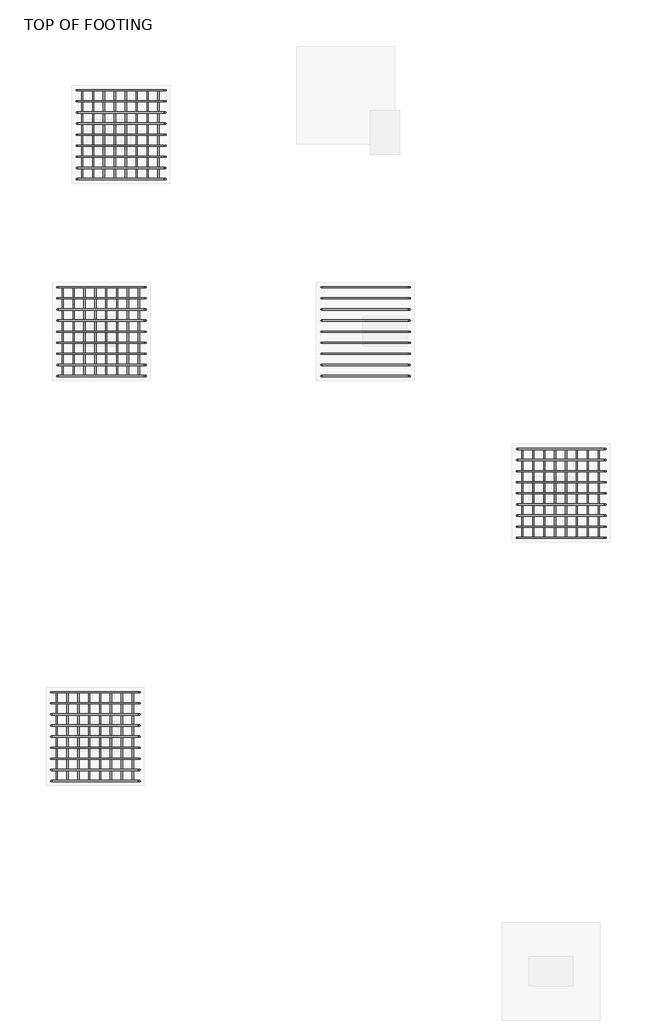
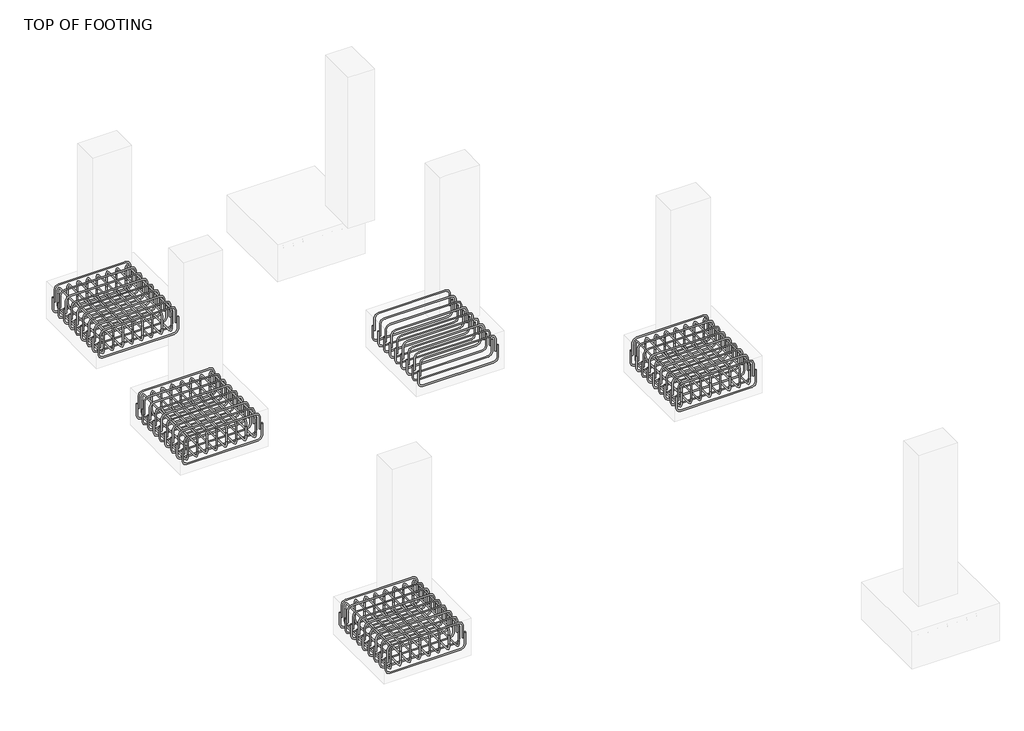
# One storey, part 15 of 20: 18 reinforcing bars.
"""IFC4 building model written with IfcOpenShell, lengths in millimetres."""

from ifc_helpers import new_model, si_unit, point, frame, origin, place, context, project, spatial, polyline, circle_curve, trimmed, segment, composite_curve, source, transform, mapped, element, save
from ifc_brep_helpers import swept_disk

model = new_model("IFC4")

# Units and contexts
model_context = context("Model", 3, world=origin())
ifc_project = project(units=[si_unit("LENGTHUNIT", "METRE", prefix="MILLI")], contexts=[model_context])

# Site, building, storey
site = spatial("IfcSite", under=ifc_project)
building = spatial("IfcBuilding", under=site)
storey = spatial("IfcBuildingStorey", under=building, Name="TOP OF FOOTING", Elevation=-1828.8)

# Reinforcing bars
placement = place(None, origin())
reinforcing_bar_shape = source(origin(), model_context, "Body", "SolidModel", [
    swept_disk(composite_curve([segment(polyline([(10522.7663908, 7703.3576276, -2006.6587682), (10522.7663908, 7703.3576276, -2153.9587682)]), True, "CONTINUOUS"), segment(trimmed(circle_curve(frame((10476.4163908, 7703.3576276, -2153.9587682), z_axis=(0.0, 1.0, 0.0), x_axis=(46.350000000000364, 0.0, 0.0)), 46.35), [point((10522.7663908, 7703.3576276, -2153.9587682))], [point((10476.4163908, 7703.3576276, -2200.3087682))], True, "CARTESIAN"), True, "CONTINUOUS"), segment(polyline([(10476.4163908, 7703.3576276, -2200.3087682), (9661.8163908, 7703.3576276, -2200.3087682)]), True, "CONTINUOUS"), segment(trimmed(circle_curve(frame((9661.8163908, 7703.3576276, -2153.9587682), z_axis=(0.0, 1.0, 0.0), x_axis=(0.0, 0.0, -46.34999999999991)), 46.35), [point((9661.8163908, 7703.3576276, -2200.3087682))], [point((9615.4663908, 7703.3576276, -2153.9587682))], True, "CARTESIAN"), True, "CONTINUOUS"), segment(polyline([(9615.4663908, 7703.3576276, -2153.9587682), (9615.4663908, 7703.3576276, -2006.6587682)]), True, "CONTINUOUS")], self_intersect=False), 6.35),
])
element("IfcReinforcingBar", 1, at=placement, inside=storey, context=model_context, shape_type="MappedRepresentation", body=[
    mapped(reinforcing_bar_shape, transform((0.0, 0.0, 0.0), x_axis=(1.0, 0.0, 0.0), y_axis=(0.0, 1.0, 0.0), z_axis=(0.0, 0.0, 1.0))),
    mapped(reinforcing_bar_shape, transform((0.0, -113.4125, 0.0), x_axis=(1.0, 0.0, 0.0), y_axis=(0.0, 1.0, 0.0), z_axis=(0.0, 0.0, 1.0))),
    mapped(reinforcing_bar_shape, transform((0.0, -226.825, 0.0), x_axis=(1.0, 0.0, 0.0), y_axis=(0.0, 1.0, 0.0), z_axis=(0.0, 0.0, 1.0))),
    mapped(reinforcing_bar_shape, transform((0.0, -340.2375, 0.0), x_axis=(1.0, 0.0, 0.0), y_axis=(0.0, 1.0, 0.0), z_axis=(0.0, 0.0, 1.0))),
    mapped(reinforcing_bar_shape, transform((0.0, -453.65, 0.0), x_axis=(1.0, 0.0, 0.0), y_axis=(0.0, 1.0, 0.0), z_axis=(0.0, 0.0, 1.0))),
    mapped(reinforcing_bar_shape, transform((0.0, -567.0625, 0.0), x_axis=(1.0, 0.0, 0.0), y_axis=(0.0, 1.0, 0.0), z_axis=(0.0, 0.0, 1.0))),
    mapped(reinforcing_bar_shape, transform((0.0, -680.475, 0.0), x_axis=(1.0, 0.0, 0.0), y_axis=(0.0, 1.0, 0.0), z_axis=(0.0, 0.0, 1.0))),
    mapped(reinforcing_bar_shape, transform((0.0, -793.8875, 0.0), x_axis=(1.0, 0.0, 0.0), y_axis=(0.0, 1.0, 0.0), z_axis=(0.0, 0.0, 1.0))),
    mapped(reinforcing_bar_shape, transform((0.0, -907.3, 0.0), x_axis=(1.0, 0.0, 0.0), y_axis=(0.0, 1.0, 0.0), z_axis=(0.0, 0.0, 1.0))),
])
reinforcing_bar_2_shape = source(origin(), model_context, "Body", "SolidModel", [
    swept_disk(composite_curve([segment(polyline([(9634.9405021, 7703.3576276, -2068.8), (9634.9405021, 7703.3576276, -1921.5)]), True, "CONTINUOUS"), segment(trimmed(circle_curve(frame((9681.2905021, 7703.3576276, -1921.5), z_axis=(0.0, 1.0, 0.0), x_axis=(-46.350000000000364, 0.0, 0.0)), 46.35), [point((9634.9405021, 7703.3576276, -1921.5))], [point((9681.2905021, 7703.3576276, -1875.15))], True, "CARTESIAN"), True, "CONTINUOUS"), segment(polyline([(9681.2905021, 7703.3576276, -1875.15), (10450.7539017, 7703.3576276, -1875.15)]), True, "CONTINUOUS"), segment(trimmed(circle_curve(frame((10450.7539017, 7703.3576276, -1921.5), z_axis=(0.0, 1.0, 0.0), x_axis=(0.0, 0.0, 46.34999999999991)), 46.35), [point((10450.7539017, 7703.3576276, -1875.15))], [point((10497.1039017, 7703.3576276, -1921.5))], True, "CARTESIAN"), True, "CONTINUOUS"), segment(polyline([(10497.1039017, 7703.3576276, -1921.5), (10497.1039017, 7703.3576276, -2068.8)]), True, "CONTINUOUS")], self_intersect=False), 6.35),
])
element("IfcReinforcingBar", 2, at=placement, inside=storey, context=model_context, shape_type="MappedRepresentation", body=[
    mapped(reinforcing_bar_2_shape, transform((0.0, 0.0, 0.0), x_axis=(1.0, 0.0, 0.0), y_axis=(0.0, 1.0, 0.0), z_axis=(0.0, 0.0, 1.0))),
    mapped(reinforcing_bar_2_shape, transform((0.0, -113.4125, 0.0), x_axis=(1.0, 0.0, 0.0), y_axis=(0.0, 1.0, 0.0), z_axis=(0.0, 0.0, 1.0))),
    mapped(reinforcing_bar_2_shape, transform((0.0, -226.825, 0.0), x_axis=(1.0, 0.0, 0.0), y_axis=(0.0, 1.0, 0.0), z_axis=(0.0, 0.0, 1.0))),
    mapped(reinforcing_bar_2_shape, transform((0.0, -340.2375, 0.0), x_axis=(1.0, 0.0, 0.0), y_axis=(0.0, 1.0, 0.0), z_axis=(0.0, 0.0, 1.0))),
    mapped(reinforcing_bar_2_shape, transform((0.0, -453.65, 0.0), x_axis=(1.0, 0.0, 0.0), y_axis=(0.0, 1.0, 0.0), z_axis=(0.0, 0.0, 1.0))),
    mapped(reinforcing_bar_2_shape, transform((0.0, -567.0625, 0.0), x_axis=(1.0, 0.0, 0.0), y_axis=(0.0, 1.0, 0.0), z_axis=(0.0, 0.0, 1.0))),
    mapped(reinforcing_bar_2_shape, transform((0.0, -680.475, 0.0), x_axis=(1.0, 0.0, 0.0), y_axis=(0.0, 1.0, 0.0), z_axis=(0.0, 0.0, 1.0))),
    mapped(reinforcing_bar_2_shape, transform((0.0, -793.8875, 0.0), x_axis=(1.0, 0.0, 0.0), y_axis=(0.0, 1.0, 0.0), z_axis=(0.0, 0.0, 1.0))),
    mapped(reinforcing_bar_2_shape, transform((0.0, -907.3, 0.0), x_axis=(1.0, 0.0, 0.0), y_axis=(0.0, 1.0, 0.0), z_axis=(0.0, 0.0, 1.0))),
])
reinforcing_bar_3_shape = source(origin(), model_context, "Body", "SolidModel", [
    swept_disk(composite_curve([segment(polyline([(10451.2694294, 7703.3576276, -2086.1951968), (10451.2694294, 7703.3576276, -1938.8951968)]), True, "CONTINUOUS"), segment(trimmed(circle_curve(frame((10451.2694294, 7657.0076276, -1938.8951968), z_axis=(1.0, 0.0, 0.0), x_axis=(0.0, 46.350000000000364, 0.0)), 46.35), [point((10451.2694294, 7703.3576276, -1938.8951968))], [point((10451.2694294, 7657.0076276, -1892.5451968))], True, "CARTESIAN"), True, "CONTINUOUS"), segment(polyline([(10451.2694294, 7657.0076276, -1892.5451968), (10451.2694294, 6842.4076276, -1892.5451968)]), True, "CONTINUOUS"), segment(trimmed(circle_curve(frame((10451.2694294, 6842.4076276, -1938.8951968), z_axis=(1.0, 0.0, 0.0), x_axis=(0.0, 0.0, 46.34999999999991)), 46.35), [point((10451.2694294, 6842.4076276, -1892.5451968))], [point((10451.2694294, 6796.0576276, -1938.8951968))], True, "CARTESIAN"), True, "CONTINUOUS"), segment(polyline([(10451.2694294, 6796.0576276, -1938.8951968), (10451.2694294, 6796.0576276, -2086.1951968)]), True, "CONTINUOUS")], self_intersect=False), 6.35),
])
element("IfcReinforcingBar", 3, at=placement, inside=storey, context=model_context, shape_type="MappedRepresentation", body=[
    mapped(reinforcing_bar_3_shape, transform((0.0, 0.0, 0.0), x_axis=(1.0, 0.0, 0.0), y_axis=(0.0, 1.0, 0.0), z_axis=(0.0, 0.0, 1.0))),
    mapped(reinforcing_bar_3_shape, transform((-111.2862402, 0.0, 0.0), x_axis=(1.0, 0.0, 0.0), y_axis=(0.0, 1.0, 0.0), z_axis=(0.0, 0.0, 1.0))),
    mapped(reinforcing_bar_3_shape, transform((-222.5724804, 0.0, 0.0), x_axis=(1.0, 0.0, 0.0), y_axis=(0.0, 1.0, 0.0), z_axis=(0.0, 0.0, 1.0))),
    mapped(reinforcing_bar_3_shape, transform((-333.8587205, 0.0, 0.0), x_axis=(1.0, 0.0, 0.0), y_axis=(0.0, 1.0, 0.0), z_axis=(0.0, 0.0, 1.0))),
    mapped(reinforcing_bar_3_shape, transform((-445.1449607, 0.0, 0.0), x_axis=(1.0, 0.0, 0.0), y_axis=(0.0, 1.0, 0.0), z_axis=(0.0, 0.0, 1.0))),
    mapped(reinforcing_bar_3_shape, transform((-556.4312009, 0.0, 0.0), x_axis=(1.0, 0.0, 0.0), y_axis=(0.0, 1.0, 0.0), z_axis=(0.0, 0.0, 1.0))),
    mapped(reinforcing_bar_3_shape, transform((-667.7174411, 0.0, 0.0), x_axis=(1.0, 0.0, 0.0), y_axis=(0.0, 1.0, 0.0), z_axis=(0.0, 0.0, 1.0))),
    mapped(reinforcing_bar_3_shape, transform((-779.0036813, 0.0, 0.0), x_axis=(1.0, 0.0, 0.0), y_axis=(0.0, 1.0, 0.0), z_axis=(0.0, 0.0, 1.0))),
])
reinforcing_bar_4_shape = source(origin(), model_context, "Body", "SolidModel", [
    swept_disk(composite_curve([segment(polyline([(9672.2657481, 7703.3576276, -1979.1645013), (9672.2657481, 7703.3576276, -2126.4645013)]), True, "CONTINUOUS"), segment(trimmed(circle_curve(frame((9672.2657481, 7657.0076276, -2126.4645013), z_axis=(-1.0, 0.0, 0.0), x_axis=(0.0, 46.350000000000364, 0.0)), 46.35), [point((9672.2657481, 7703.3576276, -2126.4645013))], [point((9672.2657481, 7657.0076276, -2172.8145013))], True, "CARTESIAN"), True, "CONTINUOUS"), segment(polyline([(9672.2657481, 7657.0076276, -2172.8145013), (9672.2657481, 6842.4076276, -2172.8145013)]), True, "CONTINUOUS"), segment(trimmed(circle_curve(frame((9672.2657481, 6842.4076276, -2126.4645013), z_axis=(-1.0, 0.0, 0.0), x_axis=(0.0, 0.0, -46.34999999999991)), 46.35), [point((9672.2657481, 6842.4076276, -2172.8145013))], [point((9672.2657481, 6796.0576276, -2126.4645013))], True, "CARTESIAN"), True, "CONTINUOUS"), segment(polyline([(9672.2657481, 6796.0576276, -2126.4645013), (9672.2657481, 6796.0576276, -1979.1645013)]), True, "CONTINUOUS")], self_intersect=False), 6.35),
])
element("IfcReinforcingBar", 4, at=placement, inside=storey, context=model_context, shape_type="MappedRepresentation", body=[
    mapped(reinforcing_bar_4_shape, transform((0.0, 0.0, 0.0), x_axis=(1.0, 0.0, 0.0), y_axis=(0.0, 1.0, 0.0), z_axis=(0.0, 0.0, 1.0))),
    mapped(reinforcing_bar_4_shape, transform((111.2862402, 0.0, 0.0), x_axis=(1.0, 0.0, 0.0), y_axis=(0.0, 1.0, 0.0), z_axis=(0.0, 0.0, 1.0))),
    mapped(reinforcing_bar_4_shape, transform((222.5724804, 0.0, 0.0), x_axis=(1.0, 0.0, 0.0), y_axis=(0.0, 1.0, 0.0), z_axis=(0.0, 0.0, 1.0))),
    mapped(reinforcing_bar_4_shape, transform((333.8587205, 0.0, 0.0), x_axis=(1.0, 0.0, 0.0), y_axis=(0.0, 1.0, 0.0), z_axis=(0.0, 0.0, 1.0))),
    mapped(reinforcing_bar_4_shape, transform((445.1449607, 0.0, 0.0), x_axis=(1.0, 0.0, 0.0), y_axis=(0.0, 1.0, 0.0), z_axis=(0.0, 0.0, 1.0))),
    mapped(reinforcing_bar_4_shape, transform((556.4312009, 0.0, 0.0), x_axis=(1.0, 0.0, 0.0), y_axis=(0.0, 1.0, 0.0), z_axis=(0.0, 0.0, 1.0))),
    mapped(reinforcing_bar_4_shape, transform((667.7174411, 0.0, 0.0), x_axis=(1.0, 0.0, 0.0), y_axis=(0.0, 1.0, 0.0), z_axis=(0.0, 0.0, 1.0))),
    mapped(reinforcing_bar_4_shape, transform((779.0036813, 0.0, 0.0), x_axis=(1.0, 0.0, 0.0), y_axis=(0.0, 1.0, 0.0), z_axis=(0.0, 0.0, 1.0))),
])
reinforcing_bar_5_shape = source(origin(), model_context, "Body", "SolidModel", [
    swept_disk(composite_curve([segment(polyline([(13022.7663908, 5691.2557249, -2006.6587682), (13022.7663908, 5691.2557249, -2153.9587682)]), True, "CONTINUOUS"), segment(trimmed(circle_curve(frame((12976.4163908, 5691.2557249, -2153.9587682), z_axis=(0.0, 1.0, 0.0), x_axis=(46.350000000000364, 0.0, 0.0)), 46.35), [point((13022.7663908, 5691.2557249, -2153.9587682))], [point((12976.4163908, 5691.2557249, -2200.3087682))], True, "CARTESIAN"), True, "CONTINUOUS"), segment(polyline([(12976.4163908, 5691.2557249, -2200.3087682), (12161.8163908, 5691.2557249, -2200.3087682)]), True, "CONTINUOUS"), segment(trimmed(circle_curve(frame((12161.8163908, 5691.2557249, -2153.9587682), z_axis=(0.0, 1.0, 0.0), x_axis=(0.0, 0.0, -46.34999999999991)), 46.35), [point((12161.8163908, 5691.2557249, -2200.3087682))], [point((12115.4663908, 5691.2557249, -2153.9587682))], True, "CARTESIAN"), True, "CONTINUOUS"), segment(polyline([(12115.4663908, 5691.2557249, -2153.9587682), (12115.4663908, 5691.2557249, -2006.6587682)]), True, "CONTINUOUS")], self_intersect=False), 6.35),
])
element("IfcReinforcingBar", 5, at=placement, inside=storey, context=model_context, shape_type="MappedRepresentation", body=[
    mapped(reinforcing_bar_5_shape, transform((0.0, 0.0, 0.0), x_axis=(1.0, 0.0, 0.0), y_axis=(0.0, 1.0, 0.0), z_axis=(0.0, 0.0, 1.0))),
    mapped(reinforcing_bar_5_shape, transform((0.0, -113.4125, 0.0), x_axis=(1.0, 0.0, 0.0), y_axis=(0.0, 1.0, 0.0), z_axis=(0.0, 0.0, 1.0))),
    mapped(reinforcing_bar_5_shape, transform((0.0, -226.825, 0.0), x_axis=(1.0, 0.0, 0.0), y_axis=(0.0, 1.0, 0.0), z_axis=(0.0, 0.0, 1.0))),
    mapped(reinforcing_bar_5_shape, transform((0.0, -340.2375, 0.0), x_axis=(1.0, 0.0, 0.0), y_axis=(0.0, 1.0, 0.0), z_axis=(0.0, 0.0, 1.0))),
    mapped(reinforcing_bar_5_shape, transform((0.0, -453.65, 0.0), x_axis=(1.0, 0.0, 0.0), y_axis=(0.0, 1.0, 0.0), z_axis=(0.0, 0.0, 1.0))),
    mapped(reinforcing_bar_5_shape, transform((0.0, -567.0625, 0.0), x_axis=(1.0, 0.0, 0.0), y_axis=(0.0, 1.0, 0.0), z_axis=(0.0, 0.0, 1.0))),
    mapped(reinforcing_bar_5_shape, transform((0.0, -680.475, 0.0), x_axis=(1.0, 0.0, 0.0), y_axis=(0.0, 1.0, 0.0), z_axis=(0.0, 0.0, 1.0))),
    mapped(reinforcing_bar_5_shape, transform((0.0, -793.8875, 0.0), x_axis=(1.0, 0.0, 0.0), y_axis=(0.0, 1.0, 0.0), z_axis=(0.0, 0.0, 1.0))),
    mapped(reinforcing_bar_5_shape, transform((0.0, -907.3, 0.0), x_axis=(1.0, 0.0, 0.0), y_axis=(0.0, 1.0, 0.0), z_axis=(0.0, 0.0, 1.0))),
])
reinforcing_bar_6_shape = source(origin(), model_context, "Body", "SolidModel", [
    swept_disk(composite_curve([segment(polyline([(12134.9405021, 5691.2557249, -2068.8), (12134.9405021, 5691.2557249, -1921.5)]), True, "CONTINUOUS"), segment(trimmed(circle_curve(frame((12181.2905021, 5691.2557249, -1921.5), z_axis=(0.0, 1.0, 0.0), x_axis=(-46.350000000000364, 0.0, 0.0)), 46.35), [point((12134.9405021, 5691.2557249, -1921.5))], [point((12181.2905021, 5691.2557249, -1875.15))], True, "CARTESIAN"), True, "CONTINUOUS"), segment(polyline([(12181.2905021, 5691.2557249, -1875.15), (12950.7539017, 5691.2557249, -1875.15)]), True, "CONTINUOUS"), segment(trimmed(circle_curve(frame((12950.7539017, 5691.2557249, -1921.5), z_axis=(0.0, 1.0, 0.0), x_axis=(0.0, 0.0, 46.34999999999991)), 46.35), [point((12950.7539017, 5691.2557249, -1875.15))], [point((12997.1039017, 5691.2557249, -1921.5))], True, "CARTESIAN"), True, "CONTINUOUS"), segment(polyline([(12997.1039017, 5691.2557249, -1921.5), (12997.1039017, 5691.2557249, -2068.8)]), True, "CONTINUOUS")], self_intersect=False), 6.35),
])
element("IfcReinforcingBar", 6, at=placement, inside=storey, context=model_context, shape_type="MappedRepresentation", body=[
    mapped(reinforcing_bar_6_shape, transform((0.0, 0.0, 0.0), x_axis=(1.0, 0.0, 0.0), y_axis=(0.0, 1.0, 0.0), z_axis=(0.0, 0.0, 1.0))),
    mapped(reinforcing_bar_6_shape, transform((0.0, -113.4125, 0.0), x_axis=(1.0, 0.0, 0.0), y_axis=(0.0, 1.0, 0.0), z_axis=(0.0, 0.0, 1.0))),
    mapped(reinforcing_bar_6_shape, transform((0.0, -226.825, 0.0), x_axis=(1.0, 0.0, 0.0), y_axis=(0.0, 1.0, 0.0), z_axis=(0.0, 0.0, 1.0))),
    mapped(reinforcing_bar_6_shape, transform((0.0, -340.2375, 0.0), x_axis=(1.0, 0.0, 0.0), y_axis=(0.0, 1.0, 0.0), z_axis=(0.0, 0.0, 1.0))),
    mapped(reinforcing_bar_6_shape, transform((0.0, -453.65, 0.0), x_axis=(1.0, 0.0, 0.0), y_axis=(0.0, 1.0, 0.0), z_axis=(0.0, 0.0, 1.0))),
    mapped(reinforcing_bar_6_shape, transform((0.0, -567.0625, 0.0), x_axis=(1.0, 0.0, 0.0), y_axis=(0.0, 1.0, 0.0), z_axis=(0.0, 0.0, 1.0))),
    mapped(reinforcing_bar_6_shape, transform((0.0, -680.475, 0.0), x_axis=(1.0, 0.0, 0.0), y_axis=(0.0, 1.0, 0.0), z_axis=(0.0, 0.0, 1.0))),
    mapped(reinforcing_bar_6_shape, transform((0.0, -793.8875, 0.0), x_axis=(1.0, 0.0, 0.0), y_axis=(0.0, 1.0, 0.0), z_axis=(0.0, 0.0, 1.0))),
    mapped(reinforcing_bar_6_shape, transform((0.0, -907.3, 0.0), x_axis=(1.0, 0.0, 0.0), y_axis=(0.0, 1.0, 0.0), z_axis=(0.0, 0.0, 1.0))),
])
reinforcing_bar_7_shape = source(origin(), model_context, "Body", "SolidModel", [
    swept_disk(composite_curve([segment(polyline([(10322.7663908, 5691.2557249, -2006.6587682), (10322.7663908, 5691.2557249, -2153.9587682)]), True, "CONTINUOUS"), segment(trimmed(circle_curve(frame((10276.4163908, 5691.2557249, -2153.9587682), z_axis=(0.0, 1.0, 0.0), x_axis=(46.350000000000364, 0.0, 0.0)), 46.35), [point((10322.7663908, 5691.2557249, -2153.9587682))], [point((10276.4163908, 5691.2557249, -2200.3087682))], True, "CARTESIAN"), True, "CONTINUOUS"), segment(polyline([(10276.4163908, 5691.2557249, -2200.3087682), (9461.8163908, 5691.2557249, -2200.3087682)]), True, "CONTINUOUS"), segment(trimmed(circle_curve(frame((9461.8163908, 5691.2557249, -2153.9587682), z_axis=(0.0, 1.0, 0.0), x_axis=(0.0, 0.0, -46.34999999999991)), 46.35), [point((9461.8163908, 5691.2557249, -2200.3087682))], [point((9415.4663908, 5691.2557249, -2153.9587682))], True, "CARTESIAN"), True, "CONTINUOUS"), segment(polyline([(9415.4663908, 5691.2557249, -2153.9587682), (9415.4663908, 5691.2557249, -2006.6587682)]), True, "CONTINUOUS")], self_intersect=False), 6.35),
])
element("IfcReinforcingBar", 7, at=placement, inside=storey, context=model_context, shape_type="MappedRepresentation", body=[
    mapped(reinforcing_bar_7_shape, transform((0.0, 0.0, 0.0), x_axis=(1.0, 0.0, 0.0), y_axis=(0.0, 1.0, 0.0), z_axis=(0.0, 0.0, 1.0))),
    mapped(reinforcing_bar_7_shape, transform((0.0, -113.4125, 0.0), x_axis=(1.0, 0.0, 0.0), y_axis=(0.0, 1.0, 0.0), z_axis=(0.0, 0.0, 1.0))),
    mapped(reinforcing_bar_7_shape, transform((0.0, -226.825, 0.0), x_axis=(1.0, 0.0, 0.0), y_axis=(0.0, 1.0, 0.0), z_axis=(0.0, 0.0, 1.0))),
    mapped(reinforcing_bar_7_shape, transform((0.0, -340.2375, 0.0), x_axis=(1.0, 0.0, 0.0), y_axis=(0.0, 1.0, 0.0), z_axis=(0.0, 0.0, 1.0))),
    mapped(reinforcing_bar_7_shape, transform((0.0, -453.65, 0.0), x_axis=(1.0, 0.0, 0.0), y_axis=(0.0, 1.0, 0.0), z_axis=(0.0, 0.0, 1.0))),
    mapped(reinforcing_bar_7_shape, transform((0.0, -567.0625, 0.0), x_axis=(1.0, 0.0, 0.0), y_axis=(0.0, 1.0, 0.0), z_axis=(0.0, 0.0, 1.0))),
    mapped(reinforcing_bar_7_shape, transform((0.0, -680.475, 0.0), x_axis=(1.0, 0.0, 0.0), y_axis=(0.0, 1.0, 0.0), z_axis=(0.0, 0.0, 1.0))),
    mapped(reinforcing_bar_7_shape, transform((0.0, -793.8875, 0.0), x_axis=(1.0, 0.0, 0.0), y_axis=(0.0, 1.0, 0.0), z_axis=(0.0, 0.0, 1.0))),
    mapped(reinforcing_bar_7_shape, transform((0.0, -907.3, 0.0), x_axis=(1.0, 0.0, 0.0), y_axis=(0.0, 1.0, 0.0), z_axis=(0.0, 0.0, 1.0))),
])
reinforcing_bar_8_shape = source(origin(), model_context, "Body", "SolidModel", [
    swept_disk(composite_curve([segment(polyline([(9434.9405021, 5691.2557249, -2068.8), (9434.9405021, 5691.2557249, -1921.5)]), True, "CONTINUOUS"), segment(trimmed(circle_curve(frame((9481.2905021, 5691.2557249, -1921.5), z_axis=(0.0, 1.0, 0.0), x_axis=(-46.350000000000364, 0.0, 0.0)), 46.35), [point((9434.9405021, 5691.2557249, -1921.5))], [point((9481.2905021, 5691.2557249, -1875.15))], True, "CARTESIAN"), True, "CONTINUOUS"), segment(polyline([(9481.2905021, 5691.2557249, -1875.15), (10250.7539017, 5691.2557249, -1875.15)]), True, "CONTINUOUS"), segment(trimmed(circle_curve(frame((10250.7539017, 5691.2557249, -1921.5), z_axis=(0.0, 1.0, 0.0), x_axis=(0.0, 0.0, 46.34999999999991)), 46.35), [point((10250.7539017, 5691.2557249, -1875.15))], [point((10297.1039017, 5691.2557249, -1921.5))], True, "CARTESIAN"), True, "CONTINUOUS"), segment(polyline([(10297.1039017, 5691.2557249, -1921.5), (10297.1039017, 5691.2557249, -2068.8)]), True, "CONTINUOUS")], self_intersect=False), 6.35),
])
element("IfcReinforcingBar", 8, at=placement, inside=storey, context=model_context, shape_type="MappedRepresentation", body=[
    mapped(reinforcing_bar_8_shape, transform((0.0, 0.0, 0.0), x_axis=(1.0, 0.0, 0.0), y_axis=(0.0, 1.0, 0.0), z_axis=(0.0, 0.0, 1.0))),
    mapped(reinforcing_bar_8_shape, transform((0.0, -113.4125, 0.0), x_axis=(1.0, 0.0, 0.0), y_axis=(0.0, 1.0, 0.0), z_axis=(0.0, 0.0, 1.0))),
    mapped(reinforcing_bar_8_shape, transform((0.0, -226.825, 0.0), x_axis=(1.0, 0.0, 0.0), y_axis=(0.0, 1.0, 0.0), z_axis=(0.0, 0.0, 1.0))),
    mapped(reinforcing_bar_8_shape, transform((0.0, -340.2375, 0.0), x_axis=(1.0, 0.0, 0.0), y_axis=(0.0, 1.0, 0.0), z_axis=(0.0, 0.0, 1.0))),
    mapped(reinforcing_bar_8_shape, transform((0.0, -453.65, 0.0), x_axis=(1.0, 0.0, 0.0), y_axis=(0.0, 1.0, 0.0), z_axis=(0.0, 0.0, 1.0))),
    mapped(reinforcing_bar_8_shape, transform((0.0, -567.0625, 0.0), x_axis=(1.0, 0.0, 0.0), y_axis=(0.0, 1.0, 0.0), z_axis=(0.0, 0.0, 1.0))),
    mapped(reinforcing_bar_8_shape, transform((0.0, -680.475, 0.0), x_axis=(1.0, 0.0, 0.0), y_axis=(0.0, 1.0, 0.0), z_axis=(0.0, 0.0, 1.0))),
    mapped(reinforcing_bar_8_shape, transform((0.0, -793.8875, 0.0), x_axis=(1.0, 0.0, 0.0), y_axis=(0.0, 1.0, 0.0), z_axis=(0.0, 0.0, 1.0))),
    mapped(reinforcing_bar_8_shape, transform((0.0, -907.3, 0.0), x_axis=(1.0, 0.0, 0.0), y_axis=(0.0, 1.0, 0.0), z_axis=(0.0, 0.0, 1.0))),
])
reinforcing_bar_9_shape = source(origin(), model_context, "Body", "SolidModel", [
    swept_disk(composite_curve([segment(polyline([(10251.2694294, 5691.2557249, -2086.1951968), (10251.2694294, 5691.2557249, -1938.8951968)]), True, "CONTINUOUS"), segment(trimmed(circle_curve(frame((10251.2694294, 5644.9057249, -1938.8951968), z_axis=(1.0, 0.0, 0.0), x_axis=(0.0, 46.350000000000364, 0.0)), 46.35), [point((10251.2694294, 5691.2557249, -1938.8951968))], [point((10251.2694294, 5644.9057249, -1892.5451968))], True, "CARTESIAN"), True, "CONTINUOUS"), segment(polyline([(10251.2694294, 5644.9057249, -1892.5451968), (10251.2694294, 4830.3057249, -1892.5451968)]), True, "CONTINUOUS"), segment(trimmed(circle_curve(frame((10251.2694294, 4830.3057249, -1938.8951968), z_axis=(1.0, 0.0, 0.0), x_axis=(0.0, 0.0, 46.34999999999991)), 46.35), [point((10251.2694294, 4830.3057249, -1892.5451968))], [point((10251.2694294, 4783.9557249, -1938.8951968))], True, "CARTESIAN"), True, "CONTINUOUS"), segment(polyline([(10251.2694294, 4783.9557249, -1938.8951968), (10251.2694294, 4783.9557249, -2086.1951968)]), True, "CONTINUOUS")], self_intersect=False), 6.35),
])
element("IfcReinforcingBar", 9, at=placement, inside=storey, context=model_context, shape_type="MappedRepresentation", body=[
    mapped(reinforcing_bar_9_shape, transform((0.0, 0.0, 0.0), x_axis=(1.0, 0.0, 0.0), y_axis=(0.0, 1.0, 0.0), z_axis=(0.0, 0.0, 1.0))),
    mapped(reinforcing_bar_9_shape, transform((-111.2862402, 0.0, 0.0), x_axis=(1.0, 0.0, 0.0), y_axis=(0.0, 1.0, 0.0), z_axis=(0.0, 0.0, 1.0))),
    mapped(reinforcing_bar_9_shape, transform((-222.5724804, 0.0, 0.0), x_axis=(1.0, 0.0, 0.0), y_axis=(0.0, 1.0, 0.0), z_axis=(0.0, 0.0, 1.0))),
    mapped(reinforcing_bar_9_shape, transform((-333.8587205, 0.0, 0.0), x_axis=(1.0, 0.0, 0.0), y_axis=(0.0, 1.0, 0.0), z_axis=(0.0, 0.0, 1.0))),
    mapped(reinforcing_bar_9_shape, transform((-445.1449607, 0.0, 0.0), x_axis=(1.0, 0.0, 0.0), y_axis=(0.0, 1.0, 0.0), z_axis=(0.0, 0.0, 1.0))),
    mapped(reinforcing_bar_9_shape, transform((-556.4312009, 0.0, 0.0), x_axis=(1.0, 0.0, 0.0), y_axis=(0.0, 1.0, 0.0), z_axis=(0.0, 0.0, 1.0))),
    mapped(reinforcing_bar_9_shape, transform((-667.7174411, 0.0, 0.0), x_axis=(1.0, 0.0, 0.0), y_axis=(0.0, 1.0, 0.0), z_axis=(0.0, 0.0, 1.0))),
    mapped(reinforcing_bar_9_shape, transform((-779.0036813, 0.0, 0.0), x_axis=(1.0, 0.0, 0.0), y_axis=(0.0, 1.0, 0.0), z_axis=(0.0, 0.0, 1.0))),
])
reinforcing_bar_10_shape = source(origin(), model_context, "Body", "SolidModel", [
    swept_disk(composite_curve([segment(polyline([(9472.2657481, 5691.2557249, -1979.1645013), (9472.2657481, 5691.2557249, -2126.4645013)]), True, "CONTINUOUS"), segment(trimmed(circle_curve(frame((9472.2657481, 5644.9057249, -2126.4645013), z_axis=(-1.0, 0.0, 0.0), x_axis=(0.0, 46.350000000000364, 0.0)), 46.35), [point((9472.2657481, 5691.2557249, -2126.4645013))], [point((9472.2657481, 5644.9057249, -2172.8145013))], True, "CARTESIAN"), True, "CONTINUOUS"), segment(polyline([(9472.2657481, 5644.9057249, -2172.8145013), (9472.2657481, 4830.3057249, -2172.8145013)]), True, "CONTINUOUS"), segment(trimmed(circle_curve(frame((9472.2657481, 4830.3057249, -2126.4645013), z_axis=(-1.0, 0.0, 0.0), x_axis=(0.0, 0.0, -46.34999999999991)), 46.35), [point((9472.2657481, 4830.3057249, -2172.8145013))], [point((9472.2657481, 4783.9557249, -2126.4645013))], True, "CARTESIAN"), True, "CONTINUOUS"), segment(polyline([(9472.2657481, 4783.9557249, -2126.4645013), (9472.2657481, 4783.9557249, -1979.1645013)]), True, "CONTINUOUS")], self_intersect=False), 6.35),
])
element("IfcReinforcingBar", 10, at=placement, inside=storey, context=model_context, shape_type="MappedRepresentation", body=[
    mapped(reinforcing_bar_10_shape, transform((0.0, 0.0, 0.0), x_axis=(1.0, 0.0, 0.0), y_axis=(0.0, 1.0, 0.0), z_axis=(0.0, 0.0, 1.0))),
    mapped(reinforcing_bar_10_shape, transform((111.2862402, 0.0, 0.0), x_axis=(1.0, 0.0, 0.0), y_axis=(0.0, 1.0, 0.0), z_axis=(0.0, 0.0, 1.0))),
    mapped(reinforcing_bar_10_shape, transform((222.5724804, 0.0, 0.0), x_axis=(1.0, 0.0, 0.0), y_axis=(0.0, 1.0, 0.0), z_axis=(0.0, 0.0, 1.0))),
    mapped(reinforcing_bar_10_shape, transform((333.8587205, 0.0, 0.0), x_axis=(1.0, 0.0, 0.0), y_axis=(0.0, 1.0, 0.0), z_axis=(0.0, 0.0, 1.0))),
    mapped(reinforcing_bar_10_shape, transform((445.1449607, 0.0, 0.0), x_axis=(1.0, 0.0, 0.0), y_axis=(0.0, 1.0, 0.0), z_axis=(0.0, 0.0, 1.0))),
    mapped(reinforcing_bar_10_shape, transform((556.4312009, 0.0, 0.0), x_axis=(1.0, 0.0, 0.0), y_axis=(0.0, 1.0, 0.0), z_axis=(0.0, 0.0, 1.0))),
    mapped(reinforcing_bar_10_shape, transform((667.7174411, 0.0, 0.0), x_axis=(1.0, 0.0, 0.0), y_axis=(0.0, 1.0, 0.0), z_axis=(0.0, 0.0, 1.0))),
    mapped(reinforcing_bar_10_shape, transform((779.0036813, 0.0, 0.0), x_axis=(1.0, 0.0, 0.0), y_axis=(0.0, 1.0, 0.0), z_axis=(0.0, 0.0, 1.0))),
])
reinforcing_bar_11_shape = source(origin(), model_context, "Body", "SolidModel", [
    swept_disk(composite_curve([segment(polyline([(15022.7663908, 4039.4036525, -2006.6587682), (15022.7663908, 4039.4036525, -2153.9587682)]), True, "CONTINUOUS"), segment(trimmed(circle_curve(frame((14976.4163908, 4039.4036525, -2153.9587682), z_axis=(0.0, 1.0, 0.0), x_axis=(46.350000000000364, 0.0, 0.0)), 46.35), [point((15022.7663908, 4039.4036525, -2153.9587682))], [point((14976.4163908, 4039.4036525, -2200.3087682))], True, "CARTESIAN"), True, "CONTINUOUS"), segment(polyline([(14976.4163908, 4039.4036525, -2200.3087682), (14161.8163908, 4039.4036525, -2200.3087682)]), True, "CONTINUOUS"), segment(trimmed(circle_curve(frame((14161.8163908, 4039.4036525, -2153.9587682), z_axis=(0.0, 1.0, 0.0), x_axis=(0.0, 0.0, -46.34999999999991)), 46.35), [point((14161.8163908, 4039.4036525, -2200.3087682))], [point((14115.4663908, 4039.4036525, -2153.9587682))], True, "CARTESIAN"), True, "CONTINUOUS"), segment(polyline([(14115.4663908, 4039.4036525, -2153.9587682), (14115.4663908, 4039.4036525, -2006.6587682)]), True, "CONTINUOUS")], self_intersect=False), 6.35),
])
element("IfcReinforcingBar", 11, at=placement, inside=storey, context=model_context, shape_type="MappedRepresentation", body=[
    mapped(reinforcing_bar_11_shape, transform((0.0, 0.0, 0.0), x_axis=(1.0, 0.0, 0.0), y_axis=(0.0, 1.0, 0.0), z_axis=(0.0, 0.0, 1.0))),
    mapped(reinforcing_bar_11_shape, transform((0.0, -113.4125, 0.0), x_axis=(1.0, 0.0, 0.0), y_axis=(0.0, 1.0, 0.0), z_axis=(0.0, 0.0, 1.0))),
    mapped(reinforcing_bar_11_shape, transform((0.0, -226.825, 0.0), x_axis=(1.0, 0.0, 0.0), y_axis=(0.0, 1.0, 0.0), z_axis=(0.0, 0.0, 1.0))),
    mapped(reinforcing_bar_11_shape, transform((0.0, -340.2375, 0.0), x_axis=(1.0, 0.0, 0.0), y_axis=(0.0, 1.0, 0.0), z_axis=(0.0, 0.0, 1.0))),
    mapped(reinforcing_bar_11_shape, transform((0.0, -453.65, 0.0), x_axis=(1.0, 0.0, 0.0), y_axis=(0.0, 1.0, 0.0), z_axis=(0.0, 0.0, 1.0))),
    mapped(reinforcing_bar_11_shape, transform((0.0, -567.0625, 0.0), x_axis=(1.0, 0.0, 0.0), y_axis=(0.0, 1.0, 0.0), z_axis=(0.0, 0.0, 1.0))),
    mapped(reinforcing_bar_11_shape, transform((0.0, -680.475, 0.0), x_axis=(1.0, 0.0, 0.0), y_axis=(0.0, 1.0, 0.0), z_axis=(0.0, 0.0, 1.0))),
    mapped(reinforcing_bar_11_shape, transform((0.0, -793.8875, 0.0), x_axis=(1.0, 0.0, 0.0), y_axis=(0.0, 1.0, 0.0), z_axis=(0.0, 0.0, 1.0))),
    mapped(reinforcing_bar_11_shape, transform((0.0, -907.3, 0.0), x_axis=(1.0, 0.0, 0.0), y_axis=(0.0, 1.0, 0.0), z_axis=(0.0, 0.0, 1.0))),
])
reinforcing_bar_12_shape = source(origin(), model_context, "Body", "SolidModel", [
    swept_disk(composite_curve([segment(polyline([(14134.9405021, 4039.4036525, -2068.8), (14134.9405021, 4039.4036525, -1921.5)]), True, "CONTINUOUS"), segment(trimmed(circle_curve(frame((14181.2905021, 4039.4036525, -1921.5), z_axis=(0.0, 1.0, 0.0), x_axis=(-46.350000000000364, 0.0, 0.0)), 46.35), [point((14134.9405021, 4039.4036525, -1921.5))], [point((14181.2905021, 4039.4036525, -1875.15))], True, "CARTESIAN"), True, "CONTINUOUS"), segment(polyline([(14181.2905021, 4039.4036525, -1875.15), (14950.7539017, 4039.4036525, -1875.15)]), True, "CONTINUOUS"), segment(trimmed(circle_curve(frame((14950.7539017, 4039.4036525, -1921.5), z_axis=(0.0, 1.0, 0.0), x_axis=(0.0, 0.0, 46.34999999999991)), 46.35), [point((14950.7539017, 4039.4036525, -1875.15))], [point((14997.1039017, 4039.4036525, -1921.5))], True, "CARTESIAN"), True, "CONTINUOUS"), segment(polyline([(14997.1039017, 4039.4036525, -1921.5), (14997.1039017, 4039.4036525, -2068.8)]), True, "CONTINUOUS")], self_intersect=False), 6.35),
])
element("IfcReinforcingBar", 12, at=placement, inside=storey, context=model_context, shape_type="MappedRepresentation", body=[
    mapped(reinforcing_bar_12_shape, transform((0.0, 0.0, 0.0), x_axis=(1.0, 0.0, 0.0), y_axis=(0.0, 1.0, 0.0), z_axis=(0.0, 0.0, 1.0))),
    mapped(reinforcing_bar_12_shape, transform((0.0, -113.4125, 0.0), x_axis=(1.0, 0.0, 0.0), y_axis=(0.0, 1.0, 0.0), z_axis=(0.0, 0.0, 1.0))),
    mapped(reinforcing_bar_12_shape, transform((0.0, -226.825, 0.0), x_axis=(1.0, 0.0, 0.0), y_axis=(0.0, 1.0, 0.0), z_axis=(0.0, 0.0, 1.0))),
    mapped(reinforcing_bar_12_shape, transform((0.0, -340.2375, 0.0), x_axis=(1.0, 0.0, 0.0), y_axis=(0.0, 1.0, 0.0), z_axis=(0.0, 0.0, 1.0))),
    mapped(reinforcing_bar_12_shape, transform((0.0, -453.65, 0.0), x_axis=(1.0, 0.0, 0.0), y_axis=(0.0, 1.0, 0.0), z_axis=(0.0, 0.0, 1.0))),
    mapped(reinforcing_bar_12_shape, transform((0.0, -567.0625, 0.0), x_axis=(1.0, 0.0, 0.0), y_axis=(0.0, 1.0, 0.0), z_axis=(0.0, 0.0, 1.0))),
    mapped(reinforcing_bar_12_shape, transform((0.0, -680.475, 0.0), x_axis=(1.0, 0.0, 0.0), y_axis=(0.0, 1.0, 0.0), z_axis=(0.0, 0.0, 1.0))),
    mapped(reinforcing_bar_12_shape, transform((0.0, -793.8875, 0.0), x_axis=(1.0, 0.0, 0.0), y_axis=(0.0, 1.0, 0.0), z_axis=(0.0, 0.0, 1.0))),
    mapped(reinforcing_bar_12_shape, transform((0.0, -907.3, 0.0), x_axis=(1.0, 0.0, 0.0), y_axis=(0.0, 1.0, 0.0), z_axis=(0.0, 0.0, 1.0))),
])
reinforcing_bar_13_shape = source(origin(), model_context, "Body", "SolidModel", [
    swept_disk(composite_curve([segment(polyline([(14951.2694294, 4039.4036525, -2086.1951968), (14951.2694294, 4039.4036525, -1938.8951968)]), True, "CONTINUOUS"), segment(trimmed(circle_curve(frame((14951.2694294, 3993.0536525, -1938.8951968), z_axis=(1.0, 0.0, 0.0), x_axis=(0.0, 46.34999999999991, 0.0)), 46.35), [point((14951.2694294, 4039.4036525, -1938.8951968))], [point((14951.2694294, 3993.0536525, -1892.5451968))], True, "CARTESIAN"), True, "CONTINUOUS"), segment(polyline([(14951.2694294, 3993.0536525, -1892.5451968), (14951.2694294, 3178.4536525, -1892.5451968)]), True, "CONTINUOUS"), segment(trimmed(circle_curve(frame((14951.2694294, 3178.4536525, -1938.8951968), z_axis=(1.0, 0.0, 0.0), x_axis=(0.0, 0.0, 46.34999999999991)), 46.35), [point((14951.2694294, 3178.4536525, -1892.5451968))], [point((14951.2694294, 3132.1036525, -1938.8951968))], True, "CARTESIAN"), True, "CONTINUOUS"), segment(polyline([(14951.2694294, 3132.1036525, -1938.8951968), (14951.2694294, 3132.1036525, -2086.1951968)]), True, "CONTINUOUS")], self_intersect=False), 6.35),
])
element("IfcReinforcingBar", 13, at=placement, inside=storey, context=model_context, shape_type="MappedRepresentation", body=[
    mapped(reinforcing_bar_13_shape, transform((0.0, 0.0, 0.0), x_axis=(1.0, 0.0, 0.0), y_axis=(0.0, 1.0, 0.0), z_axis=(0.0, 0.0, 1.0))),
    mapped(reinforcing_bar_13_shape, transform((-111.2862402, 0.0, 0.0), x_axis=(1.0, 0.0, 0.0), y_axis=(0.0, 1.0, 0.0), z_axis=(0.0, 0.0, 1.0))),
    mapped(reinforcing_bar_13_shape, transform((-222.5724804, 0.0, 0.0), x_axis=(1.0, 0.0, 0.0), y_axis=(0.0, 1.0, 0.0), z_axis=(0.0, 0.0, 1.0))),
    mapped(reinforcing_bar_13_shape, transform((-333.8587205, 0.0, 0.0), x_axis=(1.0, 0.0, 0.0), y_axis=(0.0, 1.0, 0.0), z_axis=(0.0, 0.0, 1.0))),
    mapped(reinforcing_bar_13_shape, transform((-445.1449607, 0.0, 0.0), x_axis=(1.0, 0.0, 0.0), y_axis=(0.0, 1.0, 0.0), z_axis=(0.0, 0.0, 1.0))),
    mapped(reinforcing_bar_13_shape, transform((-556.4312009, 0.0, 0.0), x_axis=(1.0, 0.0, 0.0), y_axis=(0.0, 1.0, 0.0), z_axis=(0.0, 0.0, 1.0))),
    mapped(reinforcing_bar_13_shape, transform((-667.7174411, 0.0, 0.0), x_axis=(1.0, 0.0, 0.0), y_axis=(0.0, 1.0, 0.0), z_axis=(0.0, 0.0, 1.0))),
    mapped(reinforcing_bar_13_shape, transform((-779.0036813, 0.0, 0.0), x_axis=(1.0, 0.0, 0.0), y_axis=(0.0, 1.0, 0.0), z_axis=(0.0, 0.0, 1.0))),
])
reinforcing_bar_14_shape = source(origin(), model_context, "Body", "SolidModel", [
    swept_disk(composite_curve([segment(polyline([(14172.2657481, 4039.4036525, -1979.1645013), (14172.2657481, 4039.4036525, -2126.4645013)]), True, "CONTINUOUS"), segment(trimmed(circle_curve(frame((14172.2657481, 3993.0536525, -2126.4645013), z_axis=(-1.0, 0.0, 0.0), x_axis=(0.0, 46.34999999999991, 0.0)), 46.35), [point((14172.2657481, 4039.4036525, -2126.4645013))], [point((14172.2657481, 3993.0536525, -2172.8145013))], True, "CARTESIAN"), True, "CONTINUOUS"), segment(polyline([(14172.2657481, 3993.0536525, -2172.8145013), (14172.2657481, 3178.4536525, -2172.8145013)]), True, "CONTINUOUS"), segment(trimmed(circle_curve(frame((14172.2657481, 3178.4536525, -2126.4645013), z_axis=(-1.0, 0.0, 0.0), x_axis=(0.0, 0.0, -46.34999999999991)), 46.35), [point((14172.2657481, 3178.4536525, -2172.8145013))], [point((14172.2657481, 3132.1036525, -2126.4645013))], True, "CARTESIAN"), True, "CONTINUOUS"), segment(polyline([(14172.2657481, 3132.1036525, -2126.4645013), (14172.2657481, 3132.1036525, -1979.1645013)]), True, "CONTINUOUS")], self_intersect=False), 6.35),
])
element("IfcReinforcingBar", 14, at=placement, inside=storey, context=model_context, shape_type="MappedRepresentation", body=[
    mapped(reinforcing_bar_14_shape, transform((0.0, 0.0, 0.0), x_axis=(1.0, 0.0, 0.0), y_axis=(0.0, 1.0, 0.0), z_axis=(0.0, 0.0, 1.0))),
    mapped(reinforcing_bar_14_shape, transform((111.2862402, 0.0, 0.0), x_axis=(1.0, 0.0, 0.0), y_axis=(0.0, 1.0, 0.0), z_axis=(0.0, 0.0, 1.0))),
    mapped(reinforcing_bar_14_shape, transform((222.5724804, 0.0, 0.0), x_axis=(1.0, 0.0, 0.0), y_axis=(0.0, 1.0, 0.0), z_axis=(0.0, 0.0, 1.0))),
    mapped(reinforcing_bar_14_shape, transform((333.8587205, 0.0, 0.0), x_axis=(1.0, 0.0, 0.0), y_axis=(0.0, 1.0, 0.0), z_axis=(0.0, 0.0, 1.0))),
    mapped(reinforcing_bar_14_shape, transform((445.1449607, 0.0, 0.0), x_axis=(1.0, 0.0, 0.0), y_axis=(0.0, 1.0, 0.0), z_axis=(0.0, 0.0, 1.0))),
    mapped(reinforcing_bar_14_shape, transform((556.4312009, 0.0, 0.0), x_axis=(1.0, 0.0, 0.0), y_axis=(0.0, 1.0, 0.0), z_axis=(0.0, 0.0, 1.0))),
    mapped(reinforcing_bar_14_shape, transform((667.7174411, 0.0, 0.0), x_axis=(1.0, 0.0, 0.0), y_axis=(0.0, 1.0, 0.0), z_axis=(0.0, 0.0, 1.0))),
    mapped(reinforcing_bar_14_shape, transform((779.0036813, 0.0, 0.0), x_axis=(1.0, 0.0, 0.0), y_axis=(0.0, 1.0, 0.0), z_axis=(0.0, 0.0, 1.0))),
])
reinforcing_bar_15_shape = source(origin(), model_context, "Body", "SolidModel", [
    swept_disk(composite_curve([segment(polyline([(10260.5179014, 1554.8213929, -2006.6587682), (10260.5179014, 1554.8213929, -2153.9587682)]), True, "CONTINUOUS"), segment(trimmed(circle_curve(frame((10214.1679014, 1554.8213929, -2153.9587682), z_axis=(0.0, 1.0, 0.0), x_axis=(46.350000000000364, 0.0, 0.0)), 46.35), [point((10260.5179014, 1554.8213929, -2153.9587682))], [point((10214.1679014, 1554.8213929, -2200.3087682))], True, "CARTESIAN"), True, "CONTINUOUS"), segment(polyline([(10214.1679014, 1554.8213929, -2200.3087682), (9399.5679014, 1554.8213929, -2200.3087682)]), True, "CONTINUOUS"), segment(trimmed(circle_curve(frame((9399.5679014, 1554.8213929, -2153.9587682), z_axis=(0.0, 1.0, 0.0), x_axis=(0.0, 0.0, -46.34999999999991)), 46.35), [point((9399.5679014, 1554.8213929, -2200.3087682))], [point((9353.2179014, 1554.8213929, -2153.9587682))], True, "CARTESIAN"), True, "CONTINUOUS"), segment(polyline([(9353.2179014, 1554.8213929, -2153.9587682), (9353.2179014, 1554.8213929, -2006.6587682)]), True, "CONTINUOUS")], self_intersect=False), 6.35),
])
element("IfcReinforcingBar", 15, at=placement, inside=storey, context=model_context, shape_type="MappedRepresentation", body=[
    mapped(reinforcing_bar_15_shape, transform((0.0, 0.0, 0.0), x_axis=(1.0, 0.0, 0.0), y_axis=(0.0, 1.0, 0.0), z_axis=(0.0, 0.0, 1.0))),
    mapped(reinforcing_bar_15_shape, transform((0.0, -113.4125, 0.0), x_axis=(1.0, 0.0, 0.0), y_axis=(0.0, 1.0, 0.0), z_axis=(0.0, 0.0, 1.0))),
    mapped(reinforcing_bar_15_shape, transform((0.0, -226.825, 0.0), x_axis=(1.0, 0.0, 0.0), y_axis=(0.0, 1.0, 0.0), z_axis=(0.0, 0.0, 1.0))),
    mapped(reinforcing_bar_15_shape, transform((0.0, -340.2375, 0.0), x_axis=(1.0, 0.0, 0.0), y_axis=(0.0, 1.0, 0.0), z_axis=(0.0, 0.0, 1.0))),
    mapped(reinforcing_bar_15_shape, transform((0.0, -453.65, 0.0), x_axis=(1.0, 0.0, 0.0), y_axis=(0.0, 1.0, 0.0), z_axis=(0.0, 0.0, 1.0))),
    mapped(reinforcing_bar_15_shape, transform((0.0, -567.0625, 0.0), x_axis=(1.0, 0.0, 0.0), y_axis=(0.0, 1.0, 0.0), z_axis=(0.0, 0.0, 1.0))),
    mapped(reinforcing_bar_15_shape, transform((0.0, -680.475, 0.0), x_axis=(1.0, 0.0, 0.0), y_axis=(0.0, 1.0, 0.0), z_axis=(0.0, 0.0, 1.0))),
    mapped(reinforcing_bar_15_shape, transform((0.0, -793.8875, 0.0), x_axis=(1.0, 0.0, 0.0), y_axis=(0.0, 1.0, 0.0), z_axis=(0.0, 0.0, 1.0))),
    mapped(reinforcing_bar_15_shape, transform((0.0, -907.3, 0.0), x_axis=(1.0, 0.0, 0.0), y_axis=(0.0, 1.0, 0.0), z_axis=(0.0, 0.0, 1.0))),
])
reinforcing_bar_16_shape = source(origin(), model_context, "Body", "SolidModel", [
    swept_disk(composite_curve([segment(polyline([(9372.6920127, 1554.8213929, -2068.8), (9372.6920127, 1554.8213929, -1921.5)]), True, "CONTINUOUS"), segment(trimmed(circle_curve(frame((9419.0420127, 1554.8213929, -1921.5), z_axis=(0.0, 1.0, 0.0), x_axis=(-46.350000000000364, 0.0, 0.0)), 46.35), [point((9372.6920127, 1554.8213929, -1921.5))], [point((9419.0420127, 1554.8213929, -1875.15))], True, "CARTESIAN"), True, "CONTINUOUS"), segment(polyline([(9419.0420127, 1554.8213929, -1875.15), (10188.5054124, 1554.8213929, -1875.15)]), True, "CONTINUOUS"), segment(trimmed(circle_curve(frame((10188.5054124, 1554.8213929, -1921.5), z_axis=(0.0, 1.0, 0.0), x_axis=(0.0, 0.0, 46.34999999999991)), 46.35), [point((10188.5054124, 1554.8213929, -1875.15))], [point((10234.8554124, 1554.8213929, -1921.5))], True, "CARTESIAN"), True, "CONTINUOUS"), segment(polyline([(10234.8554124, 1554.8213929, -1921.5), (10234.8554124, 1554.8213929, -2068.8)]), True, "CONTINUOUS")], self_intersect=False), 6.35),
])
element("IfcReinforcingBar", 16, at=placement, inside=storey, context=model_context, shape_type="MappedRepresentation", body=[
    mapped(reinforcing_bar_16_shape, transform((0.0, 0.0, 0.0), x_axis=(1.0, 0.0, 0.0), y_axis=(0.0, 1.0, 0.0), z_axis=(0.0, 0.0, 1.0))),
    mapped(reinforcing_bar_16_shape, transform((0.0, -113.4125, 0.0), x_axis=(1.0, 0.0, 0.0), y_axis=(0.0, 1.0, 0.0), z_axis=(0.0, 0.0, 1.0))),
    mapped(reinforcing_bar_16_shape, transform((0.0, -226.825, 0.0), x_axis=(1.0, 0.0, 0.0), y_axis=(0.0, 1.0, 0.0), z_axis=(0.0, 0.0, 1.0))),
    mapped(reinforcing_bar_16_shape, transform((0.0, -340.2375, 0.0), x_axis=(1.0, 0.0, 0.0), y_axis=(0.0, 1.0, 0.0), z_axis=(0.0, 0.0, 1.0))),
    mapped(reinforcing_bar_16_shape, transform((0.0, -453.65, 0.0), x_axis=(1.0, 0.0, 0.0), y_axis=(0.0, 1.0, 0.0), z_axis=(0.0, 0.0, 1.0))),
    mapped(reinforcing_bar_16_shape, transform((0.0, -567.0625, 0.0), x_axis=(1.0, 0.0, 0.0), y_axis=(0.0, 1.0, 0.0), z_axis=(0.0, 0.0, 1.0))),
    mapped(reinforcing_bar_16_shape, transform((0.0, -680.475, 0.0), x_axis=(1.0, 0.0, 0.0), y_axis=(0.0, 1.0, 0.0), z_axis=(0.0, 0.0, 1.0))),
    mapped(reinforcing_bar_16_shape, transform((0.0, -793.8875, 0.0), x_axis=(1.0, 0.0, 0.0), y_axis=(0.0, 1.0, 0.0), z_axis=(0.0, 0.0, 1.0))),
    mapped(reinforcing_bar_16_shape, transform((0.0, -907.3, 0.0), x_axis=(1.0, 0.0, 0.0), y_axis=(0.0, 1.0, 0.0), z_axis=(0.0, 0.0, 1.0))),
])
reinforcing_bar_17_shape = source(origin(), model_context, "Body", "SolidModel", [
    swept_disk(composite_curve([segment(polyline([(10189.02094, 1554.8213929, -2086.1951968), (10189.02094, 1554.8213929, -1938.8951968)]), True, "CONTINUOUS"), segment(trimmed(circle_curve(frame((10189.02094, 1508.4713929, -1938.8951968), z_axis=(1.0, 0.0, 0.0), x_axis=(0.0, 46.350000000000136, 0.0)), 46.35), [point((10189.02094, 1554.8213929, -1938.8951968))], [point((10189.02094, 1508.4713929, -1892.5451968))], True, "CARTESIAN"), True, "CONTINUOUS"), segment(polyline([(10189.02094, 1508.4713929, -1892.5451968), (10189.02094, 693.8713929, -1892.5451968)]), True, "CONTINUOUS"), segment(trimmed(circle_curve(frame((10189.02094, 693.8713929, -1938.8951968), z_axis=(1.0, 0.0, 0.0), x_axis=(0.0, 0.0, 46.34999999999991)), 46.35), [point((10189.02094, 693.8713929, -1892.5451968))], [point((10189.02094, 647.5213929, -1938.8951968))], True, "CARTESIAN"), True, "CONTINUOUS"), segment(polyline([(10189.02094, 647.5213929, -1938.8951968), (10189.02094, 647.5213929, -2086.1951968)]), True, "CONTINUOUS")], self_intersect=False), 6.35),
])
element("IfcReinforcingBar", 17, at=placement, inside=storey, context=model_context, shape_type="MappedRepresentation", body=[
    mapped(reinforcing_bar_17_shape, transform((0.0, 0.0, 0.0), x_axis=(1.0, 0.0, 0.0), y_axis=(0.0, 1.0, 0.0), z_axis=(0.0, 0.0, 1.0))),
    mapped(reinforcing_bar_17_shape, transform((-111.2862402, 0.0, 0.0), x_axis=(1.0, 0.0, 0.0), y_axis=(0.0, 1.0, 0.0), z_axis=(0.0, 0.0, 1.0))),
    mapped(reinforcing_bar_17_shape, transform((-222.5724804, 0.0, 0.0), x_axis=(1.0, 0.0, 0.0), y_axis=(0.0, 1.0, 0.0), z_axis=(0.0, 0.0, 1.0))),
    mapped(reinforcing_bar_17_shape, transform((-333.8587205, 0.0, 0.0), x_axis=(1.0, 0.0, 0.0), y_axis=(0.0, 1.0, 0.0), z_axis=(0.0, 0.0, 1.0))),
    mapped(reinforcing_bar_17_shape, transform((-445.1449607, 0.0, 0.0), x_axis=(1.0, 0.0, 0.0), y_axis=(0.0, 1.0, 0.0), z_axis=(0.0, 0.0, 1.0))),
    mapped(reinforcing_bar_17_shape, transform((-556.4312009, 0.0, 0.0), x_axis=(1.0, 0.0, 0.0), y_axis=(0.0, 1.0, 0.0), z_axis=(0.0, 0.0, 1.0))),
    mapped(reinforcing_bar_17_shape, transform((-667.7174411, 0.0, 0.0), x_axis=(1.0, 0.0, 0.0), y_axis=(0.0, 1.0, 0.0), z_axis=(0.0, 0.0, 1.0))),
    mapped(reinforcing_bar_17_shape, transform((-779.0036813, 0.0, 0.0), x_axis=(1.0, 0.0, 0.0), y_axis=(0.0, 1.0, 0.0), z_axis=(0.0, 0.0, 1.0))),
])
reinforcing_bar_18_shape = source(origin(), model_context, "Body", "SolidModel", [
    swept_disk(composite_curve([segment(polyline([(9410.0172587, 1554.8213929, -1979.1645013), (9410.0172587, 1554.8213929, -2126.4645013)]), True, "CONTINUOUS"), segment(trimmed(circle_curve(frame((9410.0172587, 1508.4713929, -2126.4645013), z_axis=(-1.0, 0.0, 0.0), x_axis=(0.0, 46.350000000000136, 0.0)), 46.35), [point((9410.0172587, 1554.8213929, -2126.4645013))], [point((9410.0172587, 1508.4713929, -2172.8145013))], True, "CARTESIAN"), True, "CONTINUOUS"), segment(polyline([(9410.0172587, 1508.4713929, -2172.8145013), (9410.0172587, 693.8713929, -2172.8145013)]), True, "CONTINUOUS"), segment(trimmed(circle_curve(frame((9410.0172587, 693.8713929, -2126.4645013), z_axis=(-1.0, 0.0, 0.0), x_axis=(0.0, 0.0, -46.34999999999991)), 46.35), [point((9410.0172587, 693.8713929, -2172.8145013))], [point((9410.0172587, 647.5213929, -2126.4645013))], True, "CARTESIAN"), True, "CONTINUOUS"), segment(polyline([(9410.0172587, 647.5213929, -2126.4645013), (9410.0172587, 647.5213929, -1979.1645013)]), True, "CONTINUOUS")], self_intersect=False), 6.35),
])
element("IfcReinforcingBar", 18, at=placement, inside=storey, context=model_context, shape_type="MappedRepresentation", body=[
    mapped(reinforcing_bar_18_shape, transform((0.0, 0.0, 0.0), x_axis=(1.0, 0.0, 0.0), y_axis=(0.0, 1.0, 0.0), z_axis=(0.0, 0.0, 1.0))),
    mapped(reinforcing_bar_18_shape, transform((111.2862402, 0.0, 0.0), x_axis=(1.0, 0.0, 0.0), y_axis=(0.0, 1.0, 0.0), z_axis=(0.0, 0.0, 1.0))),
    mapped(reinforcing_bar_18_shape, transform((222.5724804, 0.0, 0.0), x_axis=(1.0, 0.0, 0.0), y_axis=(0.0, 1.0, 0.0), z_axis=(0.0, 0.0, 1.0))),
    mapped(reinforcing_bar_18_shape, transform((333.8587205, 0.0, 0.0), x_axis=(1.0, 0.0, 0.0), y_axis=(0.0, 1.0, 0.0), z_axis=(0.0, 0.0, 1.0))),
    mapped(reinforcing_bar_18_shape, transform((445.1449607, 0.0, 0.0), x_axis=(1.0, 0.0, 0.0), y_axis=(0.0, 1.0, 0.0), z_axis=(0.0, 0.0, 1.0))),
    mapped(reinforcing_bar_18_shape, transform((556.4312009, 0.0, 0.0), x_axis=(1.0, 0.0, 0.0), y_axis=(0.0, 1.0, 0.0), z_axis=(0.0, 0.0, 1.0))),
    mapped(reinforcing_bar_18_shape, transform((667.7174411, 0.0, 0.0), x_axis=(1.0, 0.0, 0.0), y_axis=(0.0, 1.0, 0.0), z_axis=(0.0, 0.0, 1.0))),
    mapped(reinforcing_bar_18_shape, transform((779.0036813, 0.0, 0.0), x_axis=(1.0, 0.0, 0.0), y_axis=(0.0, 1.0, 0.0), z_axis=(0.0, 0.0, 1.0))),
])

save(model, "model.ifc")

# Revit data of these elements
# Elements 1, 2, 3, 4, 5, 6, 7, 8, 9, 10, 11, 12, 13, 14, 15, 16, 17, 18 (IfcReinforcingBar)
#   Phase Created = New Construction
